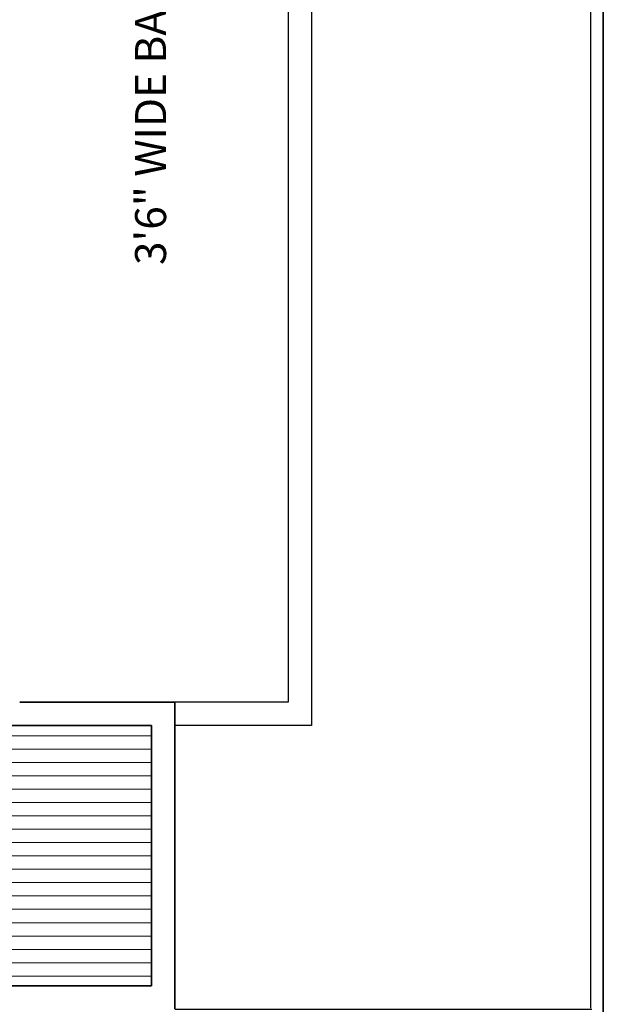
# Model space of a CAD drawing. Units: inches. Extents: x 1088 to 1703, y 668 to 1875.
# Tile 32 of 45: x 1590 to 1703, y 1416 to 1606. Entities that reach past the tile are written whole.
import ezdxf

# ---------------------------------------------------------------- set-up
doc = ezdxf.new("R2010")
doc.units = ezdxf.units.IN
for name, color, linetype, lineweight in [('A-ANNO-DIMS', 2, 'Continuous', 18), ('A-ANNO-TTLB', 7, 'Continuous', 35), ('A-AREA-IDEN', 7, 'Continuous', 18), ('A-FLOR-HRAL', 7, 'Continuous', 25), ('A-FLOR-PATT', 252, 'Continuous', 13), ('A-WALL', 7, 'Continuous', 35)]:
    doc.layers.add(name, color=color, linetype=linetype, lineweight=lineweight)
doc.styles.get("Standard").update_dxf_attribs({"font": 'arial.ttf'})
doc.dimstyles.get("Standard").update_dxf_attribs({"dimtxt": 0.18, "dimasz": 0.18, "dimexe": 0.18, "dimexo": 0.0625, "dimgap": 0.09, "dimtad": 0, "dimtih": 1, "dimtoh": 1, "dimdec": 4, "dimzin": 0, "dimdsep": 46, "dimtxsty": 'Standard', "dimcen": 0.09, "dimadec": 0, "dimazin": 0, "dimtfac": 1, "dimtdec": 4, "dimtofl": 0, "dimtmove": 0, "dimatfit": 3, "dimfxl": 1, "dimtolj": 1, "dimtzin": 0, "dimarcsym": 0})

# ---------------------------------------------------------------- blocks, each defined once
blk = doc.blocks.new('*D30')
at = {"layer": 'A-ANNO-DIMS', "color": 0, "lineweight": -2, "transparency": 16777216}
for p, q in [((1624.91, 1803.56), (1700.97, 1803.56)), ((1700.79, 1803.38), (1700.79, 1609.49)), ((1700.79, 1415.24), (1700.79, 1609.13)), ((1620.41, 1415.06), (1700.97, 1415.06))]:
    blk.add_line(p, q, dxfattribs=at)
at = {"layer": 'A-ANNO-DIMS', "color": 0, "transparency": 16777216}
for points in [[(1700.76, 1803.38), (1700.82, 1803.38), (1700.79, 1803.56)], [(1700.76, 1415.24), (1700.82, 1415.24), (1700.79, 1415.06)]]:
    blk.add_solid(points, dxfattribs=at)
at = {"layer": 'Defpoints', "color": 0, "transparency": 16777216}
for p in [(1624.84, 1803.56), (1700.79, 1803.56), (1620.34, 1415.06)]:
    blk.add_point(p, dxfattribs=at)
at = {"layer": 'A-ANNO-DIMS', "color": 0, "transparency": 16777216, "insert": (1700.79, 1609.31), "char_height": 0.18, "attachment_point": 5}
blk.add_mtext('\\A1;388.5', dxfattribs=at)

msp = doc.modelspace()

# ---------------------------------------------------------------- hatches: boundary and pattern name
at = {"layer": 'A-FLOR-PATT'}
h = msp.add_hatch(dxfattribs=at)
h.set_pattern_fill('ANSI31', color=256, scale=0.812516, angle=-45, style=0)
h.paths.add_polyline_path([(1585.845, 1419.558), (1615.845, 1419.558), (1615.845, 1469.863), (1585.845, 1469.863)])

# ---------------------------------------------------------------- linework, layer by layer
at = {"layer": 'A-ANNO-TTLB'}
msp.add_lwpolyline([(1088.369, 1874.677), (1703.181, 1874.677), (1703.181, 667.947), (1088.369, 667.947)], close=True, dxfattribs=at)
at = {"layer": 'A-FLOR-HRAL'}
for p, q in [((1646.743, 1745.49), (1646.743, 1474.363)), ((1642.243, 1740.99), (1642.243, 1474.363)), ((1642.243, 1474.363), (1620.345, 1474.363)), ((1646.743, 1474.363), (1646.743, 1469.863)), ((1646.743, 1469.863), (1620.345, 1469.863))]:
    msp.add_line(p, q, dxfattribs=at)
at = {"layer": 'A-WALL'}
for p, q in [((1620.345, 1474.363), (1590.345, 1474.363)), ((1620.345, 1415.058), (1620.345, 1474.363)), ((1615.845, 1469.863), (1585.845, 1469.863)), ((1615.845, 1469.863), (1615.845, 1419.558)), ((1615.845, 1419.558), (1585.845, 1419.558))]:
    msp.add_line(p, q, dxfattribs=at)

# ---------------------------------------------------------------- texts
at = {"layer": 'A-AREA-IDEN', "insert": (1612.649, 1558.891), "char_height": 6, "attachment_point": 1, "rotation": 90}
msp.add_mtext_dynamic_manual_height_columns('3\'6" WIDE BALCONY', width=280.65936, gutter_width=12.5, heights=[0], dxfattribs=at)

# ---------------------------------------------------------------- dimensions: what is measured, and where the dimension line sits
at = {"layer": 'A-ANNO-DIMS'}
dim = msp.add_linear_dim(base=(1700.793, 1803.558), p1=(1620.345, 1415.058), p2=(1624.845, 1803.558), angle=90, dimstyle='Standard', override={"dimdec": 1, "dimlfac": 1, "dimrnd": 0, "dimzin": 0, "dimdsep": 46, "dimlunit": 2}, dxfattribs=at)
dim.commit()
dim.dimension.update_dxf_attribs({"geometry": '*D30', "text_midpoint": (1700.793, 1609.308)})

doc.saveas('drawing.dxf')
